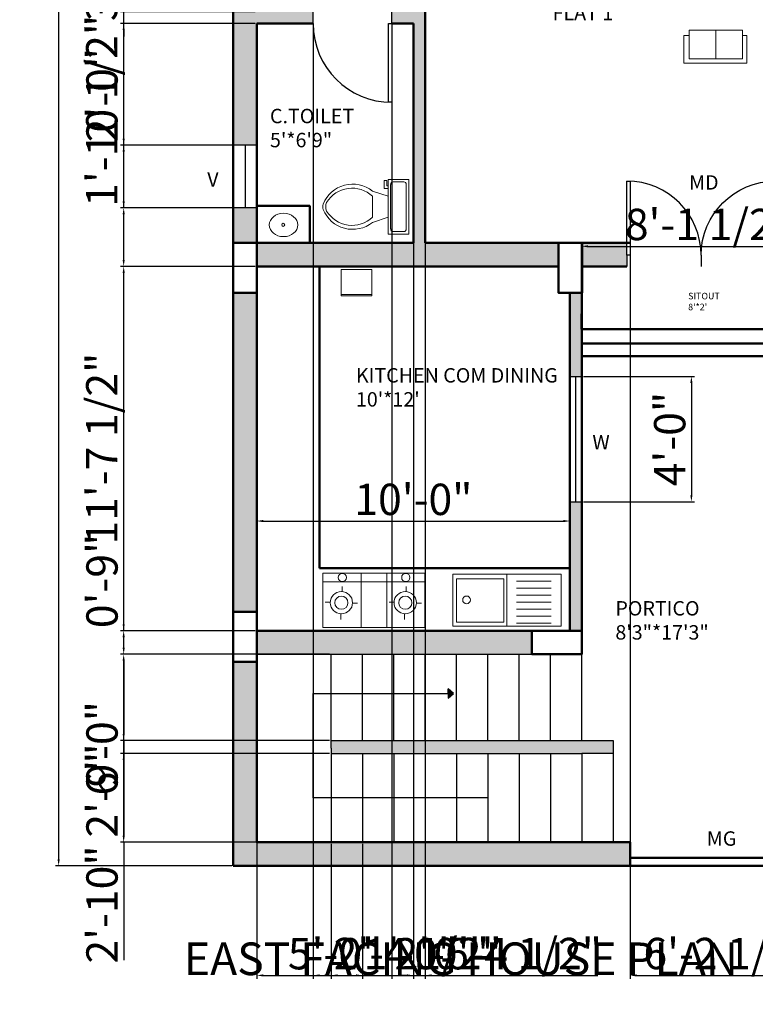
# Model space of a CAD drawing. Units: inches. Extents: x 2063 to 3370, y 2091 to 2971.
# Tile 1 of 14: x 2063 to 2345, y 2091 to 2468. Entities that reach past the tile are written whole.
import ezdxf

# ---------------------------------------------------------------- set-up
doc = ezdxf.new("R2010")
doc.units = ezdxf.units.IN
for name, color, linetype, lineweight in [('A-ANNO-DIMS', 2, 'Continuous', 18), ('A-ANNO-TEXT', 7, 'Continuous', 18), ('A-AREA-IDEN', 3, 'Continuous', 18), ('A-COLS', 7, 'Continuous', 50), ('A-DOOR', 4, 'Continuous', 25), ('A-EQPM', 8, 'Continuous', 18), ('A-FLOR-FIXT', 9, 'Continuous', 18), ('A-FLOR-STRS', 3, 'Continuous', 25), ('A-FURN', 8, 'Continuous', 18), ('A-GLAZ', 131, 'Continuous', 25), ('A-WALL', 7, 'Continuous', 50), ('A-WALL-PATT', 8, 'Continuous', 13)]:
    doc.layers.add(name, color=color, linetype=linetype, lineweight=lineweight)
doc.styles.get("Standard").update_dxf_attribs({"font": 'arial.ttf'})
doc.dimstyles.new('ISO-25', dxfattribs={"dimtxt": 12, "dimasz": 2.5, "dimexe": 1.25, "dimexo": 0.625, "dimtad": 1, "dimdec": 0, "dimlunit": 4, "dimtxsty": 'Standard', "dimcen": 2.5, "dimadec": 0, "dimazin": 0, "dimtfac": 1, "dimtdec": 0, "dimtmove": 0, "dimatfit": 3, "dimfxl": 1, "dimarcsym": 0})

# ---------------------------------------------------------------- blocks, each defined once
blk = doc.blocks.new('*U4')
for p, q in [((9.5, -6), (9.5, -2)), ((-10, -8.5), (-8, -8.5)), ((-10, -9.5), (-10, -8.5)), ((-7, -9.5), (-10, -9.5)), ((-8, -8.5), (-8, -8)), ((-7, -8), (-7, -9.5)), ((-4, -8), (-6, -14)), ((4, -8), (6, -14)), ((4, -14), (-4, -14))]:
    blk.add_line(p, q)
blk.add_lwpolyline([(10.5, -8), (10.5, 0), (-10.5, 0), (-10.5, -8)], close=True)
for points in [[(-9.5, -2), (-9.5, -6)], [(8.5, -1), (-8.5, -1)], [(-8.5, -7), (8.5, -7)]]:
    blk.add_lwpolyline(points)
for centre, radius, start, end in [((-8.62, -1.88), 0.884, 81.8699, 188.1301), ((8.62, -1.88), 0.884, 351.8699, 98.1301), ((-8.62, -6.12), 0.884, 171.8699, 278.1301), ((8.62, -6.12), 0.884, 261.8699, 8.1301), ((3.52, -21.58), 12.17, 141.4691, 247.9714), ((4.2, -21.82), 11.33, 136.3677, 238.9468), ((-3.52, -21.58), 12.17, 292.0284, 38.5307), ((-4.2, -21.82), 11.33, 301.053, 43.6321), ((0, -27.88), 4, 245.7318, 294.2682), ((0, -29), 4, 254.8605, 285.1395)]:
    blk.add_arc(centre, radius, start, end)
blk = doc.blocks.new('*U2')
for p, q in [((0, 0), (0, -6)), ((40, 0), (40, -6))]:
    blk.add_line(p, q)
blk.add_lwpolyline([(0, 0), (0, 40), (1.75, 40), (1.75, 0)], close=True)
blk.add_arc((0, 0), 40, 0, 90)
blk = doc.blocks.new('*D6')
at = {"layer": 'A-ANNO-DIMS', "color": 0, "lineweight": -2, "transparency": 16777216}
for p, q in [((2144.1, 2864.43), (2076.56, 2864.43)), ((2077.81, 2861.93), (2077.81, 2146.93)), ((2144.1, 2144.43), (2076.56, 2144.43))]:
    blk.add_line(p, q, dxfattribs=at)
at = {"layer": 'A-ANNO-DIMS', "color": 0, "transparency": 16777216}
for points in [[(2077.39, 2861.93), (2078.23, 2861.93), (2077.81, 2864.43)], [(2077.39, 2146.93), (2078.23, 2146.93), (2077.81, 2144.43)]]:
    blk.add_solid(points, dxfattribs=at)
at = {"layer": 'Defpoints', "color": 0, "transparency": 16777216}
for p in [(2144.72, 2864.43), (2077.81, 2144.43), (2144.72, 2144.43)]:
    blk.add_point(p, dxfattribs=at)
at = {"layer": 'A-ANNO-DIMS', "color": 0, "transparency": 16777216, "insert": (2071.06, 2504.43), "char_height": 12, "attachment_point": 5, "rotation": 90}
blk.add_mtext("60'", dxfattribs=at)
blk = doc.blocks.new('SOFA-2SEAT')
for p, q in [((0, 2.07), (0, 12.63)), ((0, 12.63), (24.16, 12.63)), ((24.16, 12.63), (24.16, 2.07)), ((12.27, 11.03), (12.27, 0)), ((2.08, 2.07), (0, 2.07)), ((24.16, 2.07), (22.46, 2.07))]:
    blk.add_line(p, q)
blk.add_lwpolyline([(22.46, 0), (2.08, 0), (2.08, 11.03), (22.46, 11.03)], close=True)
blk = doc.blocks.new('*D39')
at = {"layer": 'A-ANNO-DIMS', "color": 0, "lineweight": -2, "transparency": 16777216}
for p, q in [((2153.72, 2152.8), (2153.72, 2101.18)), ((2182.22, 2152.8), (2182.22, 2101.18)), ((2156.22, 2102.43), (2179.72, 2102.43)), ((2182.22, 2102.43), (2246.04, 2102.43))]:
    blk.add_line(p, q, dxfattribs=at)
at = {"layer": 'A-ANNO-DIMS', "color": 0, "transparency": 16777216}
for points in [[(2156.22, 2102.84), (2156.22, 2102.01), (2153.72, 2102.43)], [(2179.72, 2102.84), (2179.72, 2102.01), (2182.22, 2102.43)]]:
    blk.add_solid(points, dxfattribs=at)
at = {"layer": 'Defpoints', "color": 0, "transparency": 16777216}
for p in [(2153.72, 2153.43), (2182.22, 2153.43), (2182.22, 2102.43)]:
    blk.add_point(p, dxfattribs=at)
at = {"layer": 'A-ANNO-DIMS', "color": 0, "transparency": 16777216, "insert": (2215.38, 2109.26), "char_height": 12, "attachment_point": 5}
blk.add_mtext('2\'-4 1/2"', dxfattribs=at)
blk = doc.blocks.new('*D40')
at = {"layer": 'A-ANNO-DIMS', "color": 0, "lineweight": -2, "transparency": 16777216}
for p, q in [((2182.22, 2152.8), (2182.22, 2101.18)), ((2194.22, 2152.8), (2194.22, 2101.18)), ((2184.72, 2102.43), (2191.72, 2102.43)), ((2194.22, 2102.43), (2228.74, 2102.43))]:
    blk.add_line(p, q, dxfattribs=at)
at = {"layer": 'A-ANNO-DIMS', "color": 0, "transparency": 16777216}
for points in [[(2184.72, 2102.84), (2184.72, 2102.01), (2182.22, 2102.43)], [(2191.72, 2102.84), (2191.72, 2102.01), (2194.22, 2102.43)]]:
    blk.add_solid(points, dxfattribs=at)
at = {"layer": 'Defpoints', "color": 0, "transparency": 16777216}
for p in [(2182.22, 2153.43), (2194.22, 2153.43), (2194.22, 2102.43)]:
    blk.add_point(p, dxfattribs=at)
at = {"layer": 'A-ANNO-DIMS', "color": 0, "transparency": 16777216, "insert": (2212.73, 2109.18), "char_height": 12, "attachment_point": 5}
blk.add_mtext('1\'-0"', dxfattribs=at)
blk = doc.blocks.new('*D41')
at = {"layer": 'A-ANNO-DIMS', "color": 0, "lineweight": -2, "transparency": 16777216}
for p, q in [((2296.75, 2152.8), (2296.75, 2101.18)), ((2371.36, 2152.8), (2371.36, 2101.18)), ((2299.25, 2102.43), (2368.86, 2102.43))]:
    blk.add_line(p, q, dxfattribs=at)
at = {"layer": 'A-ANNO-DIMS', "color": 0, "transparency": 16777216}
for points in [[(2299.25, 2102.84), (2299.25, 2102.01), (2296.75, 2102.43)], [(2368.86, 2102.84), (2368.86, 2102.01), (2371.36, 2102.43)]]:
    blk.add_solid(points, dxfattribs=at)
at = {"layer": 'Defpoints', "color": 0, "transparency": 16777216}
for p in [(2296.75, 2153.43), (2371.36, 2153.43), (2371.36, 2102.43)]:
    blk.add_point(p, dxfattribs=at)
at = {"layer": 'A-ANNO-DIMS', "color": 0, "transparency": 16777216, "insert": (2334.06, 2109.26), "char_height": 12, "attachment_point": 5}
blk.add_mtext('6\'-2 1/2"', dxfattribs=at)
blk = doc.blocks.new('*D42')
at = {"layer": 'A-ANNO-DIMS', "color": 0, "lineweight": -2, "transparency": 16777216}
for p, q in [((2153.72, 2235.05), (2153.72, 2277.68)), ((2273.72, 2235.05), (2273.72, 2277.68)), ((2156.22, 2276.43), (2271.22, 2276.43))]:
    blk.add_line(p, q, dxfattribs=at)
at = {"layer": 'A-ANNO-DIMS', "color": 0, "transparency": 16777216}
for points in [[(2156.22, 2276.84), (2156.22, 2276.01), (2153.72, 2276.43)], [(2271.22, 2276.84), (2271.22, 2276.01), (2273.72, 2276.43)]]:
    blk.add_solid(points, dxfattribs=at)
at = {"layer": 'Defpoints', "color": 0, "transparency": 16777216}
for p in [(2273.72, 2276.43), (2153.72, 2234.43), (2273.72, 2234.43)]:
    blk.add_point(p, dxfattribs=at)
at = {"layer": 'A-ANNO-DIMS', "color": 0, "transparency": 16777216, "insert": (2213.72, 2283.18), "char_height": 12, "attachment_point": 5}
blk.add_mtext('10\'-0"', dxfattribs=at)
blk = doc.blocks.new('*D43')
at = {"layer": 'A-ANNO-DIMS', "color": 0, "lineweight": -2, "transparency": 16777216}
for p, q in [((2278.17, 2340.25), (2278.17, 2382.88)), ((2280.67, 2381.63), (2373.22, 2381.63)), ((2375.72, 2340.25), (2375.72, 2382.88))]:
    blk.add_line(p, q, dxfattribs=at)
at = {"layer": 'A-ANNO-DIMS', "color": 0, "transparency": 16777216}
for points in [[(2280.67, 2382.04), (2280.67, 2381.21), (2278.17, 2381.63)], [(2373.22, 2382.04), (2373.22, 2381.21), (2375.72, 2381.63)]]:
    blk.add_solid(points, dxfattribs=at)
at = {"layer": 'Defpoints', "color": 0, "transparency": 16777216}
for p in [(2375.72, 2381.63), (2278.17, 2339.63), (2375.72, 2339.63)]:
    blk.add_point(p, dxfattribs=at)
at = {"layer": 'A-ANNO-DIMS', "color": 0, "transparency": 16777216, "insert": (2326.95, 2388.46), "char_height": 12, "attachment_point": 5}
blk.add_mtext('8\'-1 1/2"', dxfattribs=at)
blk = doc.blocks.new('*D44')
at = {"layer": 'A-ANNO-DIMS', "color": 0, "lineweight": -2, "transparency": 16777216}
for p, q in [((2153.72, 2466.3), (2153.72, 2101.18)), ((2213.72, 2466.3), (2213.72, 2101.18)), ((2156.22, 2102.43), (2211.22, 2102.43))]:
    blk.add_line(p, q, dxfattribs=at)
at = {"layer": 'A-ANNO-DIMS', "color": 0, "transparency": 16777216}
for points in [[(2156.22, 2102.84), (2156.22, 2102.01), (2153.72, 2102.43)], [(2211.22, 2102.84), (2211.22, 2102.01), (2213.72, 2102.43)]]:
    blk.add_solid(points, dxfattribs=at)
at = {"layer": 'Defpoints', "color": 0, "transparency": 16777216}
for p in [(2153.72, 2466.93), (2213.72, 2466.93), (2213.72, 2102.43)]:
    blk.add_point(p, dxfattribs=at)
at = {"layer": 'A-ANNO-DIMS', "color": 0, "transparency": 16777216, "insert": (2183.72, 2109.18), "char_height": 12, "attachment_point": 5}
blk.add_mtext('5\'-0"', dxfattribs=at)
blk = doc.blocks.new('*D45')
at = {"layer": 'A-ANNO-DIMS', "color": 0, "lineweight": -2, "transparency": 16777216}
for p, q in [((2213.72, 2466.3), (2213.72, 2101.18)), ((2218.22, 2466.3), (2218.22, 2101.18)), ((2211.22, 2102.43), (2208.72, 2102.43)), ((2213.72, 2102.43), (2218.22, 2102.43)), ((2220.72, 2102.43), (2284.33, 2102.43))]:
    blk.add_line(p, q, dxfattribs=at)
at = {"layer": 'A-ANNO-DIMS', "color": 0, "transparency": 16777216}
for points in [[(2211.22, 2102.84), (2211.22, 2102.01), (2213.72, 2102.43)], [(2220.72, 2102.84), (2220.72, 2102.01), (2218.22, 2102.43)]]:
    blk.add_solid(points, dxfattribs=at)
at = {"layer": 'Defpoints', "color": 0, "transparency": 16777216}
for p in [(2213.72, 2466.93), (2218.22, 2466.93), (2218.22, 2102.43)]:
    blk.add_point(p, dxfattribs=at)
at = {"layer": 'A-ANNO-DIMS', "color": 0, "transparency": 16777216, "insert": (2253.78, 2109.26), "char_height": 12, "attachment_point": 5}
blk.add_mtext('0\'-4 1/2"', dxfattribs=at)
blk = doc.blocks.new('*D46')
at = {"layer": 'A-ANNO-DIMS', "color": 0, "lineweight": -2, "transparency": 16777216}
for p, q in [((2296.8, 2382.3), (2296.8, 2101.18)), ((2351.15, 2382.3), (2351.15, 2101.18)), ((2299.3, 2102.43), (2348.65, 2102.43)), ((2351.15, 2102.43), (2415.24, 2102.43))]:
    blk.add_line(p, q, dxfattribs=at)
at = {"layer": 'A-ANNO-DIMS', "color": 0, "transparency": 16777216}
for points in [[(2299.3, 2102.84), (2299.3, 2102.01), (2296.8, 2102.43)], [(2348.65, 2102.84), (2348.65, 2102.01), (2351.15, 2102.43)]]:
    blk.add_solid(points, dxfattribs=at)
at = {"layer": 'Defpoints', "color": 0, "transparency": 16777216}
for p in [(2296.8, 2382.93), (2351.15, 2382.93), (2351.15, 2102.43)]:
    blk.add_point(p, dxfattribs=at)
at = {"layer": 'A-ANNO-DIMS', "color": 0, "transparency": 16777216, "insert": (2384.45, 2109.26), "char_height": 12, "attachment_point": 5}
blk.add_mtext('4\'-6 1/2"', dxfattribs=at)
blk = doc.blocks.new('*D47')
at = {"layer": 'A-ANNO-DIMS', "color": 0, "lineweight": -2, "transparency": 16777216}
for p, q in [((2153.1, 2225.43), (2101.47, 2225.43)), ((2102.72, 2155.93), (2102.72, 2222.93)), ((2153.1, 2153.43), (2101.47, 2153.43))]:
    blk.add_line(p, q, dxfattribs=at)
at = {"layer": 'A-ANNO-DIMS', "color": 0, "transparency": 16777216}
for points in [[(2102.31, 2222.93), (2103.14, 2222.93), (2102.72, 2225.43)], [(2102.31, 2155.93), (2103.14, 2155.93), (2102.72, 2153.43)]]:
    blk.add_solid(points, dxfattribs=at)
at = {"layer": 'Defpoints', "color": 0, "transparency": 16777216}
for p in [(2102.72, 2225.43), (2153.72, 2225.43), (2153.72, 2153.43)]:
    blk.add_point(p, dxfattribs=at)
at = {"layer": 'A-ANNO-DIMS', "color": 0, "transparency": 16777216, "insert": (2095.97, 2189.43), "char_height": 12, "attachment_point": 5, "rotation": 90}
blk.add_mtext('6\'-0"', dxfattribs=at)
blk = doc.blocks.new('*D48')
at = {"layer": 'A-ANNO-DIMS', "color": 0, "lineweight": -2, "transparency": 16777216}
for p, q in [((2102.72, 2234.43), (2102.72, 2270.08)), ((2153.1, 2234.43), (2101.47, 2234.43)), ((2102.72, 2227.93), (2102.72, 2231.93)), ((2153.1, 2225.43), (2101.47, 2225.43))]:
    blk.add_line(p, q, dxfattribs=at)
at = {"layer": 'A-ANNO-DIMS', "color": 0, "transparency": 16777216}
for points in [[(2102.31, 2231.93), (2103.14, 2231.93), (2102.72, 2234.43)], [(2102.31, 2227.93), (2103.14, 2227.93), (2102.72, 2225.43)]]:
    blk.add_solid(points, dxfattribs=at)
at = {"layer": 'Defpoints', "color": 0, "transparency": 16777216}
for p in [(2102.72, 2234.43), (2153.72, 2234.43), (2153.72, 2225.43)]:
    blk.add_point(p, dxfattribs=at)
at = {"layer": 'A-ANNO-DIMS', "color": 0, "transparency": 16777216, "insert": (2095.97, 2253.5), "char_height": 12, "attachment_point": 5, "rotation": 90}
blk.add_mtext('0\'-9"', dxfattribs=at)
blk = doc.blocks.new('*D49')
at = {"layer": 'A-ANNO-DIMS', "color": 0, "lineweight": -2, "transparency": 16777216}
for p, q in [((2153.1, 2373.93), (2101.47, 2373.93)), ((2102.72, 2236.93), (2102.72, 2371.43)), ((2153.1, 2234.43), (2101.47, 2234.43))]:
    blk.add_line(p, q, dxfattribs=at)
at = {"layer": 'A-ANNO-DIMS', "color": 0, "transparency": 16777216}
for points in [[(2102.31, 2371.43), (2103.14, 2371.43), (2102.72, 2373.93)], [(2102.31, 2236.93), (2103.14, 2236.93), (2102.72, 2234.43)]]:
    blk.add_solid(points, dxfattribs=at)
at = {"layer": 'Defpoints', "color": 0, "transparency": 16777216}
for p in [(2102.72, 2373.93), (2153.72, 2373.93), (2153.72, 2234.43)]:
    blk.add_point(p, dxfattribs=at)
at = {"layer": 'A-ANNO-DIMS', "color": 0, "transparency": 16777216, "insert": (2095.89, 2304.18), "char_height": 12, "attachment_point": 5, "rotation": 90}
blk.add_mtext('11\'-7 1/2"', dxfattribs=at)
blk = doc.blocks.new('*D50')
at = {"layer": 'A-ANNO-DIMS', "color": 0, "lineweight": -2, "transparency": 16777216}
for p, q in [((2102.72, 2396.38), (2102.72, 2468.18)), ((2153.1, 2396.38), (2101.47, 2396.38)), ((2102.72, 2376.43), (2102.72, 2393.88)), ((2153.1, 2373.93), (2101.47, 2373.93))]:
    blk.add_line(p, q, dxfattribs=at)
at = {"layer": 'A-ANNO-DIMS', "color": 0, "transparency": 16777216}
for points in [[(2102.31, 2393.88), (2103.14, 2393.88), (2102.72, 2396.38)], [(2102.31, 2376.43), (2103.14, 2376.43), (2102.72, 2373.93)]]:
    blk.add_solid(points, dxfattribs=at)
at = {"layer": 'Defpoints', "color": 0, "transparency": 16777216}
for p in [(2102.72, 2396.38), (2153.72, 2396.38), (2153.72, 2373.93)]:
    blk.add_point(p, dxfattribs=at)
at = {"layer": 'A-ANNO-DIMS', "color": 0, "transparency": 16777216, "insert": (2095.89, 2433.53), "char_height": 12, "attachment_point": 5, "rotation": 90}
blk.add_mtext('1\'-10 1/2"', dxfattribs=at)
blk = doc.blocks.new('*D51')
at = {"layer": 'A-ANNO-DIMS', "color": 0, "lineweight": -2, "transparency": 16777216}
for p, q in [((2102.72, 2420.38), (2102.72, 2456.23)), ((2153.1, 2420.38), (2101.47, 2420.38)), ((2102.72, 2398.88), (2102.72, 2417.88)), ((2153.1, 2396.38), (2101.47, 2396.38))]:
    blk.add_line(p, q, dxfattribs=at)
at = {"layer": 'A-ANNO-DIMS', "color": 0, "transparency": 16777216}
for points in [[(2102.31, 2417.88), (2103.14, 2417.88), (2102.72, 2420.38)], [(2102.31, 2398.88), (2103.14, 2398.88), (2102.72, 2396.38)]]:
    blk.add_solid(points, dxfattribs=at)
at = {"layer": 'Defpoints', "color": 0, "transparency": 16777216}
for p in [(2102.72, 2420.38), (2153.72, 2420.38), (2153.72, 2396.38)]:
    blk.add_point(p, dxfattribs=at)
at = {"layer": 'A-ANNO-DIMS', "color": 0, "transparency": 16777216, "insert": (2095.97, 2439.56), "char_height": 12, "attachment_point": 5, "rotation": 90}
blk.add_mtext('2\'-0"', dxfattribs=at)
blk = doc.blocks.new('*D52')
at = {"layer": 'A-ANNO-DIMS', "color": 0, "lineweight": -2, "transparency": 16777216}
for p, q in [((2102.72, 2466.93), (2102.72, 2539.85)), ((2153.1, 2466.93), (2101.47, 2466.93)), ((2102.72, 2422.88), (2102.72, 2464.43)), ((2153.1, 2420.38), (2101.47, 2420.38))]:
    blk.add_line(p, q, dxfattribs=at)
at = {"layer": 'A-ANNO-DIMS', "color": 0, "transparency": 16777216}
for points in [[(2102.31, 2464.43), (2103.14, 2464.43), (2102.72, 2466.93)], [(2102.31, 2422.88), (2103.14, 2422.88), (2102.72, 2420.38)]]:
    blk.add_solid(points, dxfattribs=at)
at = {"layer": 'Defpoints', "color": 0, "transparency": 16777216}
for p in [(2102.72, 2466.93), (2153.72, 2466.93), (2153.72, 2420.38)]:
    blk.add_point(p, dxfattribs=at)
at = {"layer": 'A-ANNO-DIMS', "color": 0, "transparency": 16777216, "insert": (2095.89, 2504.64), "char_height": 12, "attachment_point": 5, "rotation": 90}
blk.add_mtext('3\'-10 1/2"', dxfattribs=at)
blk = doc.blocks.new('*D53')
at = {"layer": 'A-ANNO-DIMS', "color": 0, "lineweight": -2, "transparency": 16777216}
for p, q in [((2102.72, 2473.93), (2102.72, 2537.54)), ((2153.1, 2471.43), (2101.47, 2471.43)), ((2102.72, 2466.93), (2102.72, 2471.43)), ((2153.1, 2466.93), (2101.47, 2466.93)), ((2102.72, 2464.43), (2102.72, 2461.93))]:
    blk.add_line(p, q, dxfattribs=at)
at = {"layer": 'A-ANNO-DIMS', "color": 0, "transparency": 16777216}
for points in [[(2102.31, 2473.93), (2103.14, 2473.93), (2102.72, 2471.43)], [(2102.31, 2464.43), (2103.14, 2464.43), (2102.72, 2466.93)]]:
    blk.add_solid(points, dxfattribs=at)
at = {"layer": 'Defpoints', "color": 0, "transparency": 16777216}
for p in [(2102.72, 2471.43), (2153.72, 2471.43), (2153.72, 2466.93)]:
    blk.add_point(p, dxfattribs=at)
at = {"layer": 'A-ANNO-DIMS', "color": 0, "transparency": 16777216, "insert": (2095.89, 2506.98), "char_height": 12, "attachment_point": 5, "rotation": 90}
blk.add_mtext('0\'-4 1/2"', dxfattribs=at)
blk = doc.blocks.new('*D70')
at = {"layer": 'A-ANNO-DIMS', "color": 0, "lineweight": -2, "transparency": 16777216}
for p, q in [((2181.6, 2225.43), (2101.47, 2225.43)), ((2102.72, 2222.93), (2102.72, 2194.93)), ((2181.6, 2192.43), (2101.47, 2192.43)), ((2102.72, 2192.43), (2102.72, 2156.57))]:
    blk.add_line(p, q, dxfattribs=at)
at = {"layer": 'A-ANNO-DIMS', "color": 0, "transparency": 16777216}
for points in [[(2102.31, 2222.93), (2103.14, 2222.93), (2102.72, 2225.43)], [(2102.31, 2194.93), (2103.14, 2194.93), (2102.72, 2192.43)]]:
    blk.add_solid(points, dxfattribs=at)
at = {"layer": 'Defpoints', "color": 0, "transparency": 16777216}
for p in [(2182.22, 2225.43), (2102.72, 2192.43), (2182.22, 2192.43)]:
    blk.add_point(p, dxfattribs=at)
at = {"layer": 'A-ANNO-DIMS', "color": 0, "transparency": 16777216, "insert": (2095.97, 2173.25), "char_height": 12, "attachment_point": 5, "rotation": 90}
blk.add_mtext('2\'-9"', dxfattribs=at)
blk = doc.blocks.new('*D71')
at = {"layer": 'A-ANNO-DIMS', "color": 0, "lineweight": -2, "transparency": 16777216}
for p, q in [((2181.6, 2187.43), (2101.47, 2187.43)), ((2102.72, 2184.93), (2102.72, 2155.93)), ((2181.6, 2153.43), (2101.47, 2153.43)), ((2102.72, 2153.43), (2102.72, 2108.25))]:
    blk.add_line(p, q, dxfattribs=at)
at = {"layer": 'A-ANNO-DIMS', "color": 0, "transparency": 16777216}
for points in [[(2102.31, 2184.93), (2103.14, 2184.93), (2102.72, 2187.43)], [(2102.31, 2155.93), (2103.14, 2155.93), (2102.72, 2153.43)]]:
    blk.add_solid(points, dxfattribs=at)
at = {"layer": 'Defpoints', "color": 0, "transparency": 16777216}
for p in [(2182.22, 2187.43), (2102.72, 2153.43), (2182.22, 2153.43)]:
    blk.add_point(p, dxfattribs=at)
at = {"layer": 'A-ANNO-DIMS', "color": 0, "transparency": 16777216, "insert": (2095.97, 2129.59), "char_height": 12, "attachment_point": 5, "rotation": 90}
blk.add_mtext('2\'-10"', dxfattribs=at)
blk = doc.blocks.new('*D75')
at = {"layer": 'A-ANNO-DIMS', "color": 0, "lineweight": -2, "transparency": 16777216}
for p, q in [((2175.31, 2466.28), (2175.31, 2101.18)), ((2205.44, 2466.28), (2205.44, 2101.18)), ((2177.81, 2102.43), (2202.94, 2102.43)), ((2205.44, 2102.43), (2241.29, 2102.43))]:
    blk.add_line(p, q, dxfattribs=at)
at = {"layer": 'A-ANNO-DIMS', "color": 0, "transparency": 16777216}
for points in [[(2177.81, 2102.84), (2177.81, 2102.01), (2175.31, 2102.43)], [(2202.94, 2102.84), (2202.94, 2102.01), (2205.44, 2102.43)]]:
    blk.add_solid(points, dxfattribs=at)
at = {"layer": 'Defpoints', "color": 0, "transparency": 16777216}
for p in [(2175.31, 2466.91), (2205.44, 2466.91), (2205.44, 2102.43)]:
    blk.add_point(p, dxfattribs=at)
at = {"layer": 'A-ANNO-DIMS', "color": 0, "transparency": 16777216, "insert": (2224.61, 2109.18), "char_height": 12, "attachment_point": 5}
blk.add_mtext('2\'-6"', dxfattribs=at)
blk = doc.blocks.new('*D78')
at = {"layer": 'A-ANNO-DIMS', "color": 0, "lineweight": -2, "transparency": 16777216}
for p, q in [((2278.85, 2331.84), (2321.47, 2331.84)), ((2320.22, 2329.34), (2320.22, 2286.34)), ((2278.85, 2283.84), (2321.47, 2283.84))]:
    blk.add_line(p, q, dxfattribs=at)
at = {"layer": 'A-ANNO-DIMS', "color": 0, "transparency": 16777216}
for points in [[(2319.81, 2329.34), (2320.64, 2329.34), (2320.22, 2331.84)], [(2319.81, 2286.34), (2320.64, 2286.34), (2320.22, 2283.84)]]:
    blk.add_solid(points, dxfattribs=at)
at = {"layer": 'Defpoints', "color": 0, "transparency": 16777216}
for p in [(2278.22, 2331.84), (2278.22, 2283.84), (2320.22, 2283.84)]:
    blk.add_point(p, dxfattribs=at)
at = {"layer": 'A-ANNO-DIMS', "color": 0, "transparency": 16777216, "insert": (2313.47, 2307.84), "char_height": 12, "attachment_point": 5, "rotation": 90}
blk.add_mtext('4\'-0"', dxfattribs=at)

msp = doc.modelspace()

# ---------------------------------------------------------------- hatches: boundary and pattern name
at = {"layer": 'A-FLOR-STRS'}
h = msp.add_hatch(color=256, dxfattribs=at)
h.dxf.hatch_style = 1
h.paths.add_polyline_path([(2229.06, 2210.45), (2226.98, 2212.18), (2226.98, 2210.45), (2226.98, 2208.56)])
at = {"layer": 'A-WALL-PATT'}
h = msp.add_hatch(color=256, dxfattribs=at)
h.dxf.hatch_style = 1
h.paths.add_polyline_path([(2290.22, 2192.43), (2278.22, 2192.43), (2182.22, 2192.43), (2182.22, 2189.43), (2182.22, 2187.43), (2278.22, 2187.43), (2290.22, 2187.42)])
h.paths.add_polyline_path([(2748.25, 2192.43), (2736.25, 2192.43), (2640.25, 2192.43), (2640.25, 2189.43), (2640.25, 2187.43), (2736.25, 2187.43), (2748.25, 2187.42)], flags=17)
h.paths.add_polyline_path([(2653.66, 2234.43), (2611.75, 2234.43), (2611.75, 2232.93), (2611.75, 2225.43), (2653.66, 2225.43)])
h.paths.add_polyline_path([(2717.13, 2234.43), (2675.81, 2234.43), (2675.81, 2225.43), (2717.13, 2225.43)])
h.paths.add_polyline_path([(2611.75, 2222.57), (2602.75, 2222.57), (2602.75, 2144.43), (2842.75, 2144.43), (2842.75, 2220.3), (2833.75, 2220.3), (2833.75, 2153.43), (2829.39, 2153.43), (2754.78, 2153.43), (2611.75, 2153.43)])
h.paths.add_polyline_path([(2687.64, 2308.91), (2683.14, 2308.91), (2683.14, 2234.43), (2687.64, 2234.43)])
h.paths.add_polyline_path([(2744.5, 2234.43), (2736.25, 2234.43), (2736.25, 2225.43), (2744.5, 2225.43)])
h.paths.add_polyline_path([(2785.14, 2260.02), (2782.31, 2260.02), (2780.64, 2260.02), (2780.64, 2234.43), (2766.65, 2234.43), (2766.65, 2225.43), (2785.14, 2225.43)])
h.paths.add_polyline_path([(2842.75, 2363.93), (2833.75, 2363.93), (2833.75, 2239.41), (2842.75, 2239.41)])
h.paths.add_polyline_path([(2775.49, 2177.04), (2815.13, 2177.04), (2815.13, 2197.65), (2775.49, 2197.65)], flags=25)
h.paths.add_polyline_path([(2634.18, 2285.75), (2670.81, 2285.75), (2670.81, 2306.35), (2634.18, 2306.35)], flags=9)
h.paths.add_polyline_path([(2701.65, 2293.1), (2755.85, 2293.1), (2755.85, 2313.71), (2701.65, 2313.71)], flags=9)
h.paths.add_polyline_path([(2735.8, 2415.55), (2772.95, 2415.55), (2772.95, 2436.13), (2735.8, 2436.13)], flags=9)
h.paths.add_polyline_path([(2641.75, 2422.21), (2718.67, 2422.21), (2718.67, 2442.82), (2641.75, 2442.82)], flags=9)
h.paths.add_polyline_path([(2710.43, 2552.92), (2764.91, 2552.92), (2764.91, 2573.53), (2710.43, 2573.53)], flags=9)
h.paths.add_polyline_path([(2625.23, 2527.83), (2661.86, 2527.83), (2661.86, 2548.44), (2625.23, 2548.44)], flags=9)
h.paths.add_polyline_path([(2627.53, 2598.16), (2652.13, 2598.16), (2652.13, 2618.77), (2627.53, 2618.77)], flags=9)
h.paths.add_polyline_path([(2646.64, 2696.08), (2723.56, 2696.08), (2723.56, 2716.69), (2646.64, 2716.69)], flags=9)
h.paths.add_polyline_path([(2791.65, 2795.64), (2828.72, 2795.64), (2828.72, 2807.02), (2791.65, 2807.02)], flags=9)
h.paths.add_polyline_path([(2751.88, 2214.78), (2761.93, 2214.78), (2761.93, 2226.17), (2751.88, 2226.17)], flags=9)
h.paths.add_polyline_path([(2788.26, 2413.43), (2796.17, 2413.43), (2796.17, 2424.82), (2788.26, 2424.82)], flags=9)
h.paths.add_polyline_path([(2761.97, 2835.24), (2769.88, 2835.24), (2769.88, 2846.62), (2761.97, 2846.62)], flags=9)
h.paths.add_polyline_path([(2675.89, 2833.68), (2685.93, 2833.68), (2685.93, 2845.06), (2675.89, 2845.06)], flags=9)
h.paths.add_polyline_path([(2728.86, 2795.64), (2765.93, 2795.64), (2765.93, 2807.02), (2728.86, 2807.02)], flags=9)
h.paths.add_polyline_path([(2760.39, 2726.09), (2823.16, 2726.09), (2823.16, 2746.7), (2760.39, 2746.7)], flags=9)
h = msp.add_hatch(color=256, dxfattribs=at)
h.dxf.hatch_style = 1
h.paths.add_polyline_path([(2384.72, 2679.03), (2375.72, 2679.03), (2375.72, 2645.28), (2384.72, 2645.28)])
h.paths.add_polyline_path([(2384.72, 2626.16), (2375.72, 2626.16), (2375.72, 2576.43), (2327.14, 2576.43), (2327.14, 2571.93), (2375.72, 2571.93), (2375.72, 2523.93), (2384.72, 2523.93)])
h.paths.add_polyline_path([(2384.72, 2463.93), (2375.72, 2463.93), (2375.72, 2383.04), (2384.72, 2383.04)])
h.paths.add_polyline_path([(2153.72, 2812.31), (2144.72, 2812.31), (2144.72, 2638.63), (2153.72, 2638.63)])
h.paths.add_polyline_path([(2225.08, 2576.43), (2153.72, 2576.43), (2153.72, 2619.52), (2144.72, 2619.52), (2144.72, 2420.38), (2153.72, 2420.38), (2153.72, 2466.93), (2175.31, 2466.93), (2175.31, 2471.43), (2153.72, 2471.43), (2153.72, 2519.43), (2213.72, 2519.43), (2213.72, 2507.47), (2214.09, 2507.47), (2218.22, 2507.47), (2218.22, 2519.43), (2218.22, 2523.93), (2218.22, 2529.53), (2213.72, 2529.53), (2213.72, 2523.93), (2153.72, 2523.93), (2153.72, 2571.93), (2213.72, 2571.93), (2213.72, 2563.16), (2218.22, 2563.16), (2218.22, 2571.93), (2225.08, 2571.93)])
h = msp.add_hatch(color=256, dxfattribs=at)
h.dxf.hatch_style = 1
h.paths.add_polyline_path([(2269.36, 2382.93), (2218.22, 2382.93), (2218.22, 2466.93), (2218.22, 2471.43), (2218.22, 2479.94), (2213.72, 2479.94), (2213.72, 2471.43), (2205.44, 2471.43), (2205.44, 2466.93), (2213.72, 2466.93), (2213.72, 2382.93), (2153.72, 2382.93), (2153.72, 2373.93), (2269.36, 2373.93)])
h.paths.add_polyline_path([(2278.22, 2363.81), (2273.72, 2363.81), (2273.72, 2331.84), (2278.22, 2331.84)])
h.paths.add_polyline_path([(2295.55, 2382.93), (2278.36, 2382.93), (2278.36, 2373.93), (2295.55, 2373.93), (2295.55, 2378.19)])
h.paths.add_polyline_path([(2259.11, 2234.43), (2153.72, 2234.43), (2153.72, 2225.43), (2259.11, 2225.43)])
h.paths.add_polyline_path([(2278.22, 2283.84), (2273.72, 2283.84), (2273.72, 2234.43), (2278.22, 2234.43)])
h.paths.add_polyline_path([(2153.72, 2363.81), (2144.72, 2363.81), (2144.72, 2241.68), (2153.72, 2241.68)])
h = msp.add_hatch(color=256, dxfattribs=at)
h.dxf.hatch_style = 1
h.paths.add_polyline_path([(2153.72, 2222.57), (2144.72, 2222.57), (2144.72, 2144.43), (2296.75, 2144.43), (2296.75, 2153.43), (2153.72, 2153.43)])
h.paths.add_polyline_path([(2384.72, 2220.3), (2375.72, 2220.3), (2375.72, 2153.43), (2371.36, 2153.43), (2371.36, 2144.43), (2384.72, 2144.43)])
h.paths.add_polyline_path([(2384.72, 2363.93), (2375.72, 2363.93), (2375.72, 2239.41), (2384.72, 2239.41)])
h.paths.add_polyline_path([(2153.72, 2396.38), (2144.72, 2396.38), (2144.72, 2382.93), (2153.72, 2382.93)])

# ---------------------------------------------------------------- linework, layer by layer
at = {"layer": 'A-COLS'}
for points in [[(2144.72, 2382.93), (2153.72, 2382.93), (2153.72, 2363.81), (2144.72, 2363.81)], [(2269.36, 2382.93), (2278.36, 2382.93), (2278.36, 2363.81), (2269.36, 2363.81)], [(2144.72, 2241.68), (2153.72, 2241.68), (2153.72, 2222.57), (2144.72, 2222.57)], [(2259.11, 2225.43), (2259.11, 2234.43), (2278.22, 2234.43), (2278.22, 2225.43)]]:
    msp.add_lwpolyline(points, close=True, dxfattribs=at)
at = {"layer": 'A-EQPM'}
msp.add_line((2186.01, 2363.17), (2197.82, 2363.17), dxfattribs=at)
msp.add_lwpolyline([(2186.01, 2372.77), (2197.82, 2372.77), (2197.82, 2362.65), (2186.01, 2362.65)], close=True, dxfattribs=at)
at = {"layer": 'A-FLOR-FIXT'}
for p, q in [((2179.07, 2256.52), (2193.74, 2256.52)), ((2193.74, 2256.52), (2193.74, 2235.7)), ((2203.5, 2235.7), (2203.5, 2256.52)), ((2249.55, 2256.12), (2249.55, 2236.18)), ((2179.07, 2253.17), (2218.07, 2253.17)), ((2186.4, 2249.45), (2186.4, 2251.3)), ((2210.89, 2249.45), (2210.89, 2251.3)), ((2253.2, 2253.44), (2266.51, 2253.44)), ((2253.2, 2250.76), (2266.51, 2250.76)), ((2253.2, 2248.09), (2266.51, 2248.09)), ((2181.84, 2245.35), (2179.95, 2245.35)), ((2190.41, 2245.03), (2192.32, 2245.03)), ((2206.33, 2245.35), (2204.44, 2245.35)), ((2214.9, 2245.03), (2216.81, 2245.03)), ((2253.2, 2245.41), (2266.51, 2245.41)), ((2185.86, 2240.79), (2185.86, 2238.72)), ((2210.35, 2240.79), (2210.35, 2238.72)), ((2253.2, 2242.73), (2266.51, 2242.73)), ((2253.2, 2240.06), (2266.51, 2240.06)), ((2253.2, 2237.38), (2266.51, 2237.38)), ((2218.07, 2235.7), (2203.5, 2235.7))]:
    msp.add_line(p, q, dxfattribs=at)
for points in [[(2179.07, 2256.52), (2218.07, 2256.52), (2218.07, 2235.7), (2179.07, 2235.7)], [(2270.3, 2256.12), (2228.81, 2256.12), (2228.81, 2236.18), (2270.3, 2236.18)], [(2230.29, 2254.27), (2248.31, 2254.27), (2248.31, 2237.75), (2230.29, 2237.75)]]:
    msp.add_lwpolyline(points, close=True, dxfattribs=at)
for centre, radius in [((2163.85, 2389.87), 0.596), ((2186.51, 2254.83), 1.57), ((2210.8, 2254.83), 1.57), ((2186.12, 2245.17), 4.29), ((2186.12, 2245.17), 2.53), ((2210.61, 2245.17), 4.29), ((2210.61, 2245.17), 2.53), ((2234.08, 2246.24), 1.48)]:
    msp.add_circle(centre, radius, dxfattribs=at)
msp.add_ellipse((2163.97, 2389.83), major_axis=(5.46, 0), ratio=0.818182, dxfattribs=at)
at = {"layer": 'A-FLOR-STRS'}
for p, q in [((2153.72, 2225.43), (2278.22, 2225.43)), ((2182.22, 2189.43), (2182.22, 2225.43)), ((2194.22, 2192.43), (2194.22, 2225.43)), ((2206.22, 2192.43), (2206.22, 2225.43)), ((2218.22, 2192.43), (2218.22, 2225.43)), ((2230.22, 2192.43), (2230.22, 2225.43)), ((2242.22, 2192.43), (2242.22, 2225.43)), ((2254.22, 2192.43), (2254.22, 2225.43)), ((2266.22, 2192.43), (2266.22, 2225.43)), ((2278.22, 2192.43), (2278.22, 2225.43)), ((2175.36, 2170.43), (2175.36, 2210.45)), ((2175.36, 2210.45), (2226.98, 2210.45)), ((2226.98, 2210.45), (2226.98, 2212.18)), ((2229.06, 2210.45), (2226.98, 2212.18)), ((2226.98, 2210.45), (2226.98, 2208.56)), ((2226.98, 2208.56), (2229.06, 2210.45)), ((2182.22, 2192.43), (2278.22, 2192.43)), ((2290.22, 2191.04), (2290.22, 2153.43)), ((2182.22, 2189.43), (2182.22, 2153.43)), ((2182.22, 2187.43), (2278.22, 2187.43)), ((2194.22, 2187.43), (2194.22, 2153.43)), ((2206.22, 2187.43), (2206.22, 2153.43)), ((2218.22, 2187.43), (2218.22, 2153.43)), ((2230.22, 2187.43), (2230.22, 2153.43)), ((2242.22, 2187.43), (2242.22, 2153.43)), ((2254.22, 2187.43), (2254.22, 2153.43)), ((2266.22, 2187.43), (2266.22, 2153.43)), ((2278.22, 2187.43), (2278.22, 2153.43)), ((2242.22, 2170.43), (2175.36, 2170.43))]:
    msp.add_line(p, q, dxfattribs=at)
msp.add_lwpolyline([(2278.22, 2192.43), (2290.22, 2192.43), (2290.22, 2187.42), (2278.22, 2187.42), (2278.22, 2187.43)], dxfattribs=at)
at = {"layer": 'A-GLAZ'}
for p, q in [((2153.72, 2420.38), (2144.72, 2420.38)), ((2149.22, 2420.38), (2149.22, 2396.38)), ((2153.72, 2396.38), (2144.72, 2396.38)), ((2273.72, 2331.84), (2278.22, 2331.84)), ((2275.97, 2283.84), (2275.97, 2331.84)), ((2273.72, 2283.84), (2278.22, 2283.84))]:
    msp.add_line(p, q, dxfattribs=at)
at = {"layer": 'A-WALL'}
for p, q in [((2218.22, 2471.43), (2218.22, 2466.93)), ((2153.72, 2466.93), (2175.31, 2466.93)), ((2205.44, 2466.93), (2213.72, 2466.93)), ((2213.72, 2466.93), (2213.72, 2382.93)), ((2218.22, 2466.93), (2218.22, 2382.93)), ((2153.72, 2382.93), (2213.72, 2382.93)), ((2218.22, 2382.93), (2296.8, 2382.93)), ((2323.97, 2382.93), (2323.97, 2382.93)), ((2278.22, 2234.43), (2278.22, 2378.43)), ((2153.72, 2373.93), (2269.36, 2373.93)), ((2153.72, 2373.93), (2177.72, 2373.93)), ((2177.72, 2373.93), (2177.72, 2258.43)), ((2278.36, 2373.93), (2278.17, 2349.93)), ((2278.22, 2373.93), (2295.55, 2373.93)), ((2273.72, 2363.81), (2273.72, 2234.43)), ((2273.72, 2234.43), (2273.72, 2363.81)), ((2278.17, 2349.93), (2374.17, 2349.93)), ((2278.17, 2344.41), (2374.17, 2344.41)), ((2278.17, 2339.63), (2374.17, 2339.63)), ((2273.72, 2258.43), (2177.72, 2258.43)), ((2273.72, 2234.43), (2273.72, 2258.43)), ((2153.72, 2234.43), (2278.22, 2234.43)), ((2278.22, 2234.43), (2278.22, 2225.43)), ((2296.75, 2144.43), (2296.75, 2153.43))]:
    msp.add_line(p, q, dxfattribs=at)
for points in [[(2144.72, 2144.43), (2384.72, 2144.43), (2384.72, 2864.43), (2144.72, 2864.43)], [(2153.72, 2382.93), (2174, 2382.93), (2174, 2397.13), (2153.72, 2397.13)], [(2296.75, 2144.43), (2371.36, 2144.43), (2371.36, 2147.44), (2296.75, 2147.44)]]:
    msp.add_lwpolyline(points, close=True, dxfattribs=at)
for points in [[(2153.72, 2466.93), (2153.72, 2382.93)], [(2153.72, 2378.43), (2153.72, 2234.43)], [(2153.72, 2225.43), (2153.72, 2153.43), (2296.75, 2153.43)]]:
    msp.add_lwpolyline(points, dxfattribs=at)

# ---------------------------------------------------------------- block references
at = {"layer": 'A-DOOR', "xscale": 0.753161428329689, "yscale": 0.753161428329689, "zscale": 0.753161428329689, "rotation": 180}
msp.add_blockref('*U2', (2205.44, 2466.91), dxfattribs=at)
at = {"layer": 'A-DOOR', "yscale": 0.7105099264086059, "zscale": 0.7105099264086059}
for p, xscale in [((2295.55, 2378.19), 0.7105099264086059), ((2352.39, 2378.19), -0.7105099264086059)]:
    msp.add_blockref('*U2', p, dxfattribs=dict(at, xscale=xscale))
at = {"layer": 'A-FLOR-FIXT', "rotation": 270}
msp.add_blockref('*U4', (2212.01, 2396.79), dxfattribs=at)
at = {"layer": 'A-FURN', "extrusion": (0, 0, -1), "zscale": -1, "rotation": 180}
msp.add_blockref('SOFA-2SEAT', (-2317.31, 2464.45), dxfattribs=at)

# ---------------------------------------------------------------- texts
at = {"layer": 'A-ANNO-TEXT', "attachment_point": 1}
for s, width, gutter_width, heights, insert, char_height in [('FLAT 1', 106.0361, 27.61, [14.84], (2267.05, 2473.76), 5.523), ('V', 106.0361, 27.61, [0], (2134.74, 2410), 5.52), ('MD', 106.0361, 27.61, [0], (2319.35, 2408.87), 5.523), ('W', 106.0361, 27.61, [0], (2282.31, 2309.36), 5.52), ('MG', 106.0361, 27.61, [0], (2326.14, 2157.61), 5.523), ('EAST FACING HOUSE PLAN', 239.9528, 62.49, [33.82], (2125.8, 2115.04), 12.498)]:
    msp.add_mtext_dynamic_manual_height_columns(s, width=width, gutter_width=gutter_width, heights=heights, dxfattribs=dict(at, insert=insert, char_height=char_height))
at = {"layer": 'A-AREA-IDEN', "attachment_point": 1}
for s, width, gutter_width, insert, char_height in [('C.TOILET\\P5\'*6\'9"', 106.0361, 27.61, (2158.77, 2434.3), 5.523), ("SITOUT\\P8'*2'", 17.4359, 12.5, (2318.99, 2363.84), 2.5), ("KITCHEN COM DINING\\P10'*12'", 106.0361, 27.61, (2191.7, 2334.99), 5.5229), ('PORTICO\\P8\'3"*17\'3"', 106.0361, 27.61, (2291.11, 2245.77), 5.523)]:
    msp.add_mtext_dynamic_manual_height_columns(s, width=width, gutter_width=gutter_width, heights=[0], dxfattribs=dict(at, insert=insert, char_height=char_height))

# ---------------------------------------------------------------- dimensions: what is measured, and where the dimension line sits
at = {"layer": 'A-ANNO-DIMS'}
for base, p1, p2, angle, override, picture, middle in [((2077.81, 2144.43), (2144.72, 2864.43), (2144.72, 2144.43), 90, {"dimclrd": 0, "dimclre": 0, "dimclrt": 0}, '*D6', (2071.06, 2504.43)), ((2102.722, 2466.9264), (2153.722, 2420.3799), (2153.722, 2466.9264), 90, {"dimdec": 1, "dimlfac": 1, "dimrnd": 0, "dimzin": 1, "dimdsep": 46, "dimlunit": 4, "dimfrac": 2}, '*D52', (2095.8883, 2504.6394)), ((2102.72, 2471.43), (2153.72, 2466.93), (2153.72, 2471.43), 90, {"dimdec": 1, "dimlfac": 1, "dimrnd": 0, "dimzin": 1, "dimdsep": 46, "dimlunit": 4, "dimfrac": 2}, '*D53', (2095.89, 2506.98)), ((2102.722, 2396.3799), (2153.722, 2373.9264), (2153.722, 2396.3799), 90, {"dimdec": 1, "dimlfac": 1, "dimrnd": 0, "dimzin": 1, "dimdsep": 46, "dimlunit": 4, "dimfrac": 2}, '*D50', (2095.8924, 2433.5321)), ((2102.72, 2420.38), (2153.72, 2396.38), (2153.72, 2420.38), 90, {"dimdec": 1, "dimlfac": 1, "dimrnd": 0, "dimzin": 1, "dimdsep": 46, "dimlunit": 4, "dimfrac": 2}, '*D51', (2095.97, 2439.56)), ((2102.72, 2373.93), (2153.72, 2234.43), (2153.72, 2373.93), 90, {"dimdec": 1, "dimlfac": 1, "dimrnd": 0, "dimzin": 1, "dimdsep": 46, "dimlunit": 4, "dimfrac": 2}, '*D49', (2095.89, 2304.18)), ((2320.22, 2283.84), (2278.22, 2331.84), (2278.22, 2283.84), 270, {"dimdec": 1, "dimlfac": 1, "dimrnd": 0, "dimzin": 1, "dimdsep": 46, "dimlunit": 4, "dimfrac": 2}, '*D78', (2313.47, 2307.84)), ((2102.72, 2234.43), (2153.72, 2225.43), (2153.72, 2234.43), 90, {"dimdec": 1, "dimlfac": 1, "dimrnd": 0, "dimzin": 1, "dimdsep": 46, "dimlunit": 4, "dimfrac": 2}, '*D48', (2095.97, 2253.5)), ((2102.72, 2225.43), (2153.72, 2153.43), (2153.72, 2225.43), 90, {"dimdec": 1, "dimlfac": 1, "dimrnd": 0, "dimzin": 1, "dimdsep": 46, "dimlunit": 4, "dimfrac": 2}, '*D47', (2095.97, 2189.43)), ((2102.72, 2192.43), (2182.22, 2225.43), (2182.22, 2192.43), 90, {"dimdec": 1, "dimlfac": 1, "dimrnd": 0, "dimzin": 1, "dimdsep": 46, "dimlunit": 4, "dimfrac": 2}, '*D70', (2095.97, 2173.25)), ((2102.72, 2153.43), (2182.22, 2187.43), (2182.22, 2153.43), 90, {"dimdec": 1, "dimlfac": 1, "dimrnd": 0, "dimzin": 1, "dimdsep": 46, "dimlunit": 4, "dimfrac": 2}, '*D71', (2095.97, 2129.59))]:
    dim = msp.add_linear_dim(base=base, p1=p1, p2=p2, angle=angle, dimstyle='ISO-25', override=override, dxfattribs=at)
    dim.commit()
    dim.dimension.update_dxf_attribs({"geometry": picture, "text_midpoint": middle})
for base, p1, p2, picture, middle in [((2213.72, 2102.43), (2153.72, 2466.93), (2213.72, 2466.93), '*D44', (2183.72, 2109.18)), ((2205.44, 2102.43), (2175.31, 2466.91), (2205.44, 2466.91), '*D75', (2224.61, 2109.18)), ((2218.22, 2102.43), (2213.72, 2466.93), (2218.22, 2466.93), '*D45', (2253.78, 2109.26)), ((2375.722, 2381.628), (2278.1707, 2339.628), (2375.722, 2339.628), '*D43', (2326.9464, 2388.4576)), ((2351.1508, 2102.4264), (2296.7967, 2382.9264), (2351.1508, 2382.9264), '*D46', (2384.4476, 2109.2561)), ((2273.72, 2276.43), (2153.72, 2234.43), (2273.72, 2234.43), '*D42', (2213.72, 2283.18)), ((2182.22, 2102.43), (2153.72, 2153.43), (2182.22, 2153.43), '*D39', (2215.38, 2109.26)), ((2194.22, 2102.43), (2182.22, 2153.43), (2194.22, 2153.43), '*D40', (2212.73, 2109.18)), ((2371.36, 2102.43), (2296.75, 2153.43), (2371.36, 2153.43), '*D41', (2334.06, 2109.26))]:
    dim = msp.add_linear_dim(base=base, p1=p1, p2=p2, dimstyle='ISO-25', override={"dimdec": 1, "dimlfac": 1, "dimrnd": 0, "dimzin": 1, "dimdsep": 46, "dimlunit": 4, "dimfrac": 2}, dxfattribs=at)
    dim.commit()
    dim.dimension.update_dxf_attribs({"geometry": picture, "text_midpoint": middle})

doc.saveas('drawing.dxf')
